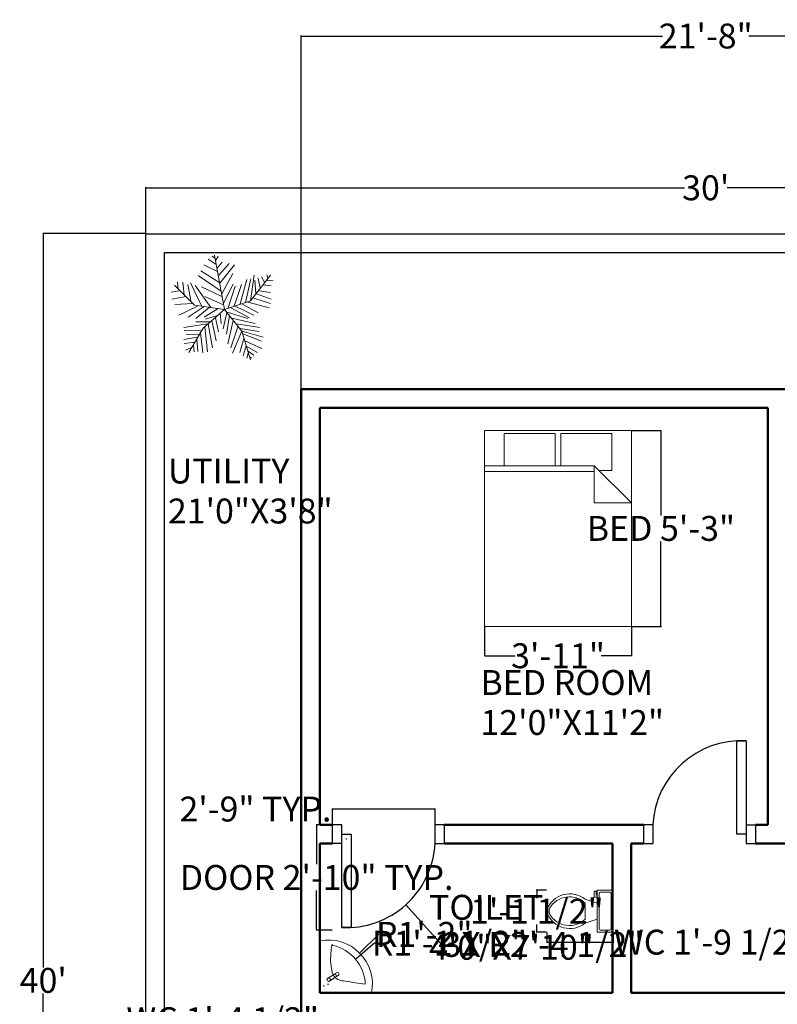
# Model space of a CAD drawing. Units: inches. Extents: x -1912 to -1462, y -785 to -198.
# Tile 2 of 3: x -1912 to -1668, y -515 to -198. Entities that reach past the tile are written whole.
import ezdxf

# ---------------------------------------------------------------- set-up
doc = ezdxf.new("R2010")
doc.units = ezdxf.units.IN
doc.header["$MEASUREMENT"] = 0
for name, color, linetype, lineweight in [('A-ANNO-DIMS', 2, 'Continuous', 18), ('A-AREA-IDEN', 7, 'Continuous', 18), ('A-DOOR', 4, 'Continuous', 25), ('A-FLOR-FIXT', 8, 'Continuous', 18), ('A-FURN', 8, 'Continuous', 18), ('A-WALL', 7, 'Continuous', 50), ('C-PROP', 8, 'Continuous', 25), ('L-PLNT-TREE', 3, 'Continuous', 13)]:
    doc.layers.add(name, color=color, linetype=linetype, lineweight=lineweight)
doc.styles.get("Standard").update_dxf_attribs({"font": 'arial.ttf'})
doc.dimstyles.get("Standard").update_dxf_attribs({"dimtxt": 8, "dimasz": 0.18, "dimexe": 0.18, "dimexo": 0.0625, "dimgap": 0.09, "dimtad": 0, "dimtih": 1, "dimtoh": 1, "dimzin": 0, "dimdsep": 46, "dimlunit": 3, "dimtxsty": 'Standard', "dimcen": 0.09, "dimadec": 0, "dimazin": 0, "dimtfac": 1, "dimtofl": 0, "dimtmove": 0, "dimatfit": 3, "dimfxl": 1, "dimtolj": 1, "dimtzin": 0, "dimarcsym": 0})

# ---------------------------------------------------------------- blocks, each defined once
blk = doc.blocks.new('Bed - Queen')
for p, q in [((0, -80.00003), (0, 0)), ((0, 0), (59.99999, 0)), ((59.99999, 0), (59.99999, -80.00003)), ((7.99999, -1.2), (28.79998, -1.2)), ((7.99999, -14.4), (7.99999, -1.2)), ((28.79998, -1.2), (28.79998, -14.4)), ((31.19999, -1.2), (51.99999, -1.2)), ((31.19999, -14.4), (31.19999, -1.2)), ((51.99999, -1.2), (51.99999, -16.4)), ((0, -14.4), (44.8, -14.4)), ((59.99999, -29.6), (44.8, -14.4)), ((44.8, -14.4), (44.8, -29.6)), ((44.8, -16.8), (0, -16.8)), ((51.99999, -16.4), (46.79936, -16.4)), ((44.8, -29.6), (59.99999, -29.6)), ((59.99999, -80.00003), (0, -80.00003))]:
    blk.add_line(p, q)
blk = doc.blocks.new('Toilet - top')
for p, q in [((9.5, -6), (9.5, -2)), ((-10, -8.5), (-8, -8.5)), ((-10, -9.5), (-10, -8.5)), ((-7, -9.5), (-10, -9.5)), ((-8, -8.5), (-8, -8)), ((-7, -8), (-7, -9.5)), ((-4, -8), (-6, -14)), ((4, -8), (6, -14)), ((4, -14), (-4, -14))]:
    blk.add_line(p, q)
blk.add_lwpolyline([(10.5, -8), (10.5, 0), (-10.5, 0), (-10.5, -8)], close=True)
for points in [[(-9.5, -2), (-9.5, -6)], [(8.5, -1), (-8.5, -1)], [(-8.5, -7), (8.5, -7)]]:
    blk.add_lwpolyline(points)
for centre, radius, start, end in [((-8.62, -1.88), 0.884, 81.8699, 188.1301), ((8.62, -1.88), 0.884, 351.8699, 98.1301), ((-8.62, -6.12), 0.884, 171.8699, 278.1301), ((8.62, -6.12), 0.884, 261.8699, 8.1301), ((3.52, -21.58), 12.17, 141.4691, 247.9714), ((4.2, -21.82), 11.33, 136.3677, 238.9468), ((-3.52, -21.58), 12.17, 292.0284, 38.5307), ((-4.2, -21.82), 11.33, 301.053, 43.6321), ((0, -27.88), 4, 245.7318, 294.2682), ((0, -29), 4, 254.8605, 285.1395)]:
    blk.add_arc(centre, radius, start, end)
blk = doc.blocks.new('*U11')
for p, q in [((-8.737, 47.138), (-17.069, 52.711)), ((-10.186, 53.64), (-13.084, 55.962)), ((0, 0), (-10.5, 57)), ((-9.099, 51.782), (-6.563, 55.962)), ((-7.288, 39.707), (-21.778, 46.673)), ((-7.65, 43.423), (-2.578, 49.46)), ((-5.839, 35.992), (4.667, 48.067)), ((-5.114, 27.632), (10.463, 46.673)), ((-3.665, 19.273), (-27.574, 35.527)), ((-5.114, 28.097), (-24.676, 40.636)), ((-2.941, 16.486), (8.652, 37.85)), ((16.259, 5.805), (23.142, 31.348)), ((22.055, 7.198), (27.489, 32.277)), ((27, 9), (48, 36)), ((27.127, 9.056), (31.112, 35.992)), ((35.096, 32.741), (37.27, 22.524)), ((38.719, 34.134), (41.979, 28.561)), ((44.153, 36.456), (45.239, 32.741)), ((-31.5, 4.5), (-52.5, 25.5)), ((-48.585, 21.131), (-49.309, 29.026)), ((-43.513, 28.561), (-42.427, 15.558)), ((-38.442, 26.239), (-34.819, 7.663)), ((-35.544, 28.097), (-24.314, 3.947)), ((-14.533, 2.09), (-30.834, 25.31)), ((-24.314, 23.917), (-2.941, 13.7)), ((-1.129, 6.734), (9.014, 26.704)), ((3.942, 1.625), (11.187, 24.381)), ((10.101, 3.483), (17.708, 26.239)), ((31.836, 30.883), (32.561, 16.486)), ((40.53, 25.775), (48.862, 24.846)), ((43.791, 29.954), (51.036, 30.883)), ((-47.498, 19.737), (-55.83, 18.344)), ((-40.615, 13.7), (-55.105, 10.913)), ((-20.691, 13.7), (-1.129, 4.876)), ((29.662, 12.307), (48.137, 6.269)), ((33.285, 16.486), (48.862, 10.913)), ((36.183, 19.737), (48.137, 17.88)), ((-33.37, 6.269), (-52.207, 5.34)), ((-28.299, 3.483), (-47.86, -5.805)), ((-21.416, 3.018), (-38.079, -8.128)), ((0, 0), (-31.5, 4.5)), ((-15.982, 2.09), (-30.11, -9.521)), ((0, 0), (-22.5, -19.5)), ((-6.563, 1.161), (-21.416, -8.128)), ((0, 0), (27, 9)), ((0, 0), (18, -22.5)), ((6.478, 1.625), (26.04, -8.592)), ((11.187, 3.483), (30.749, -5.805)), ((18.07, 5.805), (35.096, -3.483)), ((24.229, 7.663), (46.688, 1.625)), ((-6.563, -5.805), (-19.967, -9.985)), ((-9.461, -8.592), (-6.201, -23.453)), ((-4.752, -3.483), (-3.665, -14.629)), ((2.493, -3.019), (-1.491, -20.202)), ((1.769, -2.555), (24.229, -9.521)), ((5.029, -6.27), (2.131, -25.775)), ((7.565, -9.056), (32.198, -14.629)), ((-17.431, -15.094), (-42.789, -18.809)), ((-22.5, -19.5), (-37.5, -45)), ((-15.257, -12.772), (-30.11, -12.772)), ((-20.691, -18.345), (-17.793, -44.352)), ((-17.069, -15.094), (-12.721, -40.172)), ((-13.446, -11.378), (-8.737, -32.741)), ((9.014, -11.378), (3.58, -35.992)), ((14.085, -16.951), (6.478, -40.172)), ((12.274, -15.094), (36.907, -18.809)), ((16.259, -19.738), (36.183, -22.989)), ((-28.299, -29.026), (-42.789, -31.348)), ((-24.314, -21.596), (-42.427, -22.06)), ((-26.849, -26.24), (-40.253, -25.775)), ((-29.023, -30.884), (-27.936, -43.887)), ((-25.038, -23.918), (-22.865, -45.281)), ((18.07, -22.524), (8.289, -45.745)), ((20.244, -30.419), (15.897, -44.816)), ((18, -22.5), (27, -52.5)), ((18.433, -22.524), (40.53, -29.026)), ((19.157, -25.311), (38.719, -33.206)), ((-30.834, -34.135), (-42.427, -35.528)), ((-34.457, -39.708), (-40.978, -42.494)), ((-32.646, -36.921), (-31.921, -44.352)), ((22.78, -37.85), (19.519, -48.532)), ((21.331, -32.741), (39.081, -40.636)), ((22.78, -38.314), (34.372, -44.816)), ((24.591, -45.745), (23.142, -50.854)), ((24.591, -43.423), (30.749, -47.603)), ((26.764, -49.925), (28.213, -50.854))]:
    blk.add_line(p, q)
blk = doc.blocks.new('*D12')
at = {"layer": 'A-ANNO-DIMS', "color": 0, "lineweight": -2, "transparency": 16777216}
for p, q in [((-1871.08, -267.18), (-1871.08, -252.32)), ((-1870.9, -252.5), (-1697.95, -252.5)), ((-1511.26, -252.5), (-1684.2, -252.5)), ((-1511.08, -267.18), (-1511.08, -252.32))]:
    blk.add_line(p, q, dxfattribs=at)
at = {"layer": 'A-ANNO-DIMS', "color": 0, "transparency": 16777216}
for points in [[(-1870.9, -252.47), (-1870.9, -252.53), (-1871.08, -252.5)], [(-1511.26, -252.47), (-1511.26, -252.53), (-1511.08, -252.5)]]:
    blk.add_solid(points, dxfattribs=at)
at = {"layer": 'Defpoints', "color": 0, "transparency": 16777216}
for p in [(-1511.08, -252.5), (-1871.08, -267.24), (-1511.08, -267.24)]:
    blk.add_point(p, dxfattribs=at)
at = {"layer": 'A-ANNO-DIMS', "color": 0, "transparency": 16777216, "insert": (-1691.08, -252.5), "char_height": 8, "attachment_point": 5}
blk.add_mtext("\\A1;30'", dxfattribs=at)
blk = doc.blocks.new('*D13')
at = {"layer": 'A-ANNO-DIMS', "color": 0, "lineweight": -2, "transparency": 16777216}
for p, q in [((-1871.14, -267.24), (-1904.18, -267.24)), ((-1904, -267.42), (-1904, -503.07)), ((-1904, -747.06), (-1904, -511.42)), ((-1871.14, -747.24), (-1904.18, -747.24))]:
    blk.add_line(p, q, dxfattribs=at)
at = {"layer": 'A-ANNO-DIMS', "color": 0, "transparency": 16777216}
for points in [[(-1904.03, -267.42), (-1903.97, -267.42), (-1904, -267.24)], [(-1904.03, -747.06), (-1903.97, -747.06), (-1904, -747.24)]]:
    blk.add_solid(points, dxfattribs=at)
at = {"layer": 'Defpoints', "color": 0, "transparency": 16777216}
for p in [(-1871.08, -267.24), (-1904, -747.24), (-1871.08, -747.24)]:
    blk.add_point(p, dxfattribs=at)
at = {"layer": 'A-ANNO-DIMS', "color": 0, "transparency": 16777216, "insert": (-1904, -507.24), "char_height": 8, "attachment_point": 5}
blk.add_mtext("\\A1;40'", dxfattribs=at)
blk = doc.blocks.new('DOOR-30IN-LEAF-HINGE-JAMB')
for p, q in [((0, 3), (0, -3)), ((0, 3), (3, 3)), ((3, 3), (3, -3)), ((0, -3), (3, -3))]:
    blk.add_line(p, q)
blk.add_lwpolyline([(0, 0), (-3, 0), (-3, 30), (0, 30)], close=True)
blk.add_arc((-1.5, 1.5), 28.54, 86.9872, 176.9872)
blk = doc.blocks.new('*D15')
at = {"layer": 'A-ANNO-DIMS', "color": 0, "lineweight": -2, "transparency": 16777216}
for p, q in [((-1811.14, -457.24), (-1816.33, -457.24)), ((-1816.15, -457.42), (-1816.15, -469.93)), ((-1816.15, -490.89), (-1816.15, -478.38)), ((-1811.14, -491.07), (-1816.33, -491.07))]:
    blk.add_line(p, q, dxfattribs=at)
at = {"layer": 'A-ANNO-DIMS', "color": 0, "transparency": 16777216}
for points in [[(-1816.18, -457.42), (-1816.12, -457.42), (-1816.15, -457.24)], [(-1816.18, -490.89), (-1816.12, -490.89), (-1816.15, -491.07)]]:
    blk.add_solid(points, dxfattribs=at)
at = {"layer": 'Defpoints', "color": 0, "transparency": 16777216}
for p in [(-1811.08, -457.24), (-1816.15, -491.07), (-1811.08, -491.07)]:
    blk.add_point(p, dxfattribs=at)
at = {"layer": 'A-ANNO-DIMS', "color": 0, "transparency": 16777216, "insert": (-1816.15, -474.16), "char_height": 8, "attachment_point": 5}
blk.add_mtext('\\A1;DOOR 2\'-10" TYP.', dxfattribs=at)
blk = doc.blocks.new('*D16')
at = {"layer": 'A-ANNO-DIMS', "color": 0, "lineweight": -2, "transparency": 16777216}
for p, q in [((-1811.08, -452.17), (-1811.26, -452.17)), ((-1811.08, -457.18), (-1811.08, -451.99)), ((-1778.26, -452.17), (-1810.9, -452.17)), ((-1778.08, -457.18), (-1778.08, -451.99))]:
    blk.add_line(p, q, dxfattribs=at)
at = {"layer": 'A-ANNO-DIMS', "color": 0, "transparency": 16777216}
for points in [[(-1810.9, -452.14), (-1810.9, -452.2), (-1811.08, -452.17)], [(-1778.26, -452.14), (-1778.26, -452.2), (-1778.08, -452.17)]]:
    blk.add_solid(points, dxfattribs=at)
at = {"layer": 'Defpoints', "color": 0, "transparency": 16777216}
for p in [(-1811.08, -452.17), (-1811.08, -457.24), (-1778.08, -457.24)]:
    blk.add_point(p, dxfattribs=at)
at = {"layer": 'A-ANNO-DIMS', "color": 0, "transparency": 16777216, "insert": (-1835.8, -452.17), "char_height": 8, "attachment_point": 5}
blk.add_mtext('\\A1;2\'-9" TYP.', dxfattribs=at)
blk = doc.blocks.new('*D17')
at = {"layer": 'A-ANNO-DIMS', "color": 0, "lineweight": -2, "transparency": 16777216}
for p, q in [((-1742.16, -491.83), (-1742.16, -495.14)), ((-1720.86, -491.83), (-1720.86, -495.14)), ((-1741.98, -494.96), (-1721.04, -494.96)), ((-1720.86, -494.96), (-1720.68, -494.96))]:
    blk.add_line(p, q, dxfattribs=at)
at = {"layer": 'A-ANNO-DIMS', "color": 0, "transparency": 16777216}
for points in [[(-1741.98, -494.93), (-1741.98, -494.99), (-1742.16, -494.96)], [(-1721.04, -494.93), (-1721.04, -494.99), (-1720.86, -494.96)]]:
    blk.add_solid(points, dxfattribs=at)
at = {"layer": 'Defpoints', "color": 0, "transparency": 16777216}
for p in [(-1742.16, -491.77), (-1720.86, -491.77), (-1720.86, -494.96)]:
    blk.add_point(p, dxfattribs=at)
at = {"layer": 'A-ANNO-DIMS', "color": 0, "transparency": 16777216, "insert": (-1689.61, -494.96), "char_height": 8, "attachment_point": 5}
blk.add_mtext('\\A1;WC 1\'-9 1/2"', dxfattribs=at)
blk = doc.blocks.new('*D18')
at = {"layer": 'A-ANNO-DIMS', "color": 0, "lineweight": -2, "transparency": 16777216}
for p, q in [((-1742.22, -478.23), (-1745.53, -478.23)), ((-1745.35, -478.41), (-1745.35, -480.77)), ((-1745.35, -491.59), (-1745.35, -489.23)), ((-1742.22, -491.77), (-1745.53, -491.77))]:
    blk.add_line(p, q, dxfattribs=at)
at = {"layer": 'A-ANNO-DIMS', "color": 0, "transparency": 16777216}
for points in [[(-1745.38, -478.41), (-1745.32, -478.41), (-1745.35, -478.23)], [(-1745.38, -491.59), (-1745.32, -491.59), (-1745.35, -491.77)]]:
    blk.add_solid(points, dxfattribs=at)
at = {"layer": 'Defpoints', "color": 0, "transparency": 16777216}
for p in [(-1742.16, -478.23), (-1745.35, -491.77), (-1742.16, -491.77)]:
    blk.add_point(p, dxfattribs=at)
at = {"layer": 'A-ANNO-DIMS', "color": 0, "transparency": 16777216, "insert": (-1745.35, -485), "char_height": 8, "attachment_point": 5}
blk.add_mtext('\\A1;1\'-1 1/2"', dxfattribs=at)
blk = doc.blocks.new('*D19')
at = {"layer": 'A-ANNO-DIMS', "color": 0, "lineweight": -2, "transparency": 16777216}
for p, q in [((-1815.08, -519.88), (-1815.26, -519.88)), ((-1815.08, -522.26), (-1815.08, -519.7)), ((-1798.96, -519.88), (-1814.9, -519.88)), ((-1798.78, -522.26), (-1798.78, -519.7))]:
    blk.add_line(p, q, dxfattribs=at)
at = {"layer": 'A-ANNO-DIMS', "color": 0, "transparency": 16777216}
for points in [[(-1814.9, -519.85), (-1814.9, -519.91), (-1815.08, -519.88)], [(-1798.96, -519.85), (-1798.96, -519.91), (-1798.78, -519.88)]]:
    blk.add_solid(points, dxfattribs=at)
at = {"layer": 'Defpoints', "color": 0, "transparency": 16777216}
for p in [(-1815.08, -519.88), (-1815.08, -522.32), (-1798.78, -522.32)]:
    blk.add_point(p, dxfattribs=at)
at = {"layer": 'A-ANNO-DIMS', "color": 0, "transparency": 16777216, "insert": (-1846.33, -519.88), "char_height": 8, "attachment_point": 5}
blk.add_mtext('\\A1;WC 1\'-4 1/2"', dxfattribs=at)
blk = doc.blocks.new('*D29')
at = {"layer": 'A-ANNO-DIMS', "color": 0, "lineweight": -2, "transparency": 16777216}
for p, q in [((-1714.88, -330.48), (-1705.31, -330.48)), ((-1705.49, -330.66), (-1705.49, -357.79)), ((-1705.49, -393.28), (-1705.49, -366.15)), ((-1714.88, -393.46), (-1705.31, -393.46))]:
    blk.add_line(p, q, dxfattribs=at)
at = {"layer": 'A-ANNO-DIMS', "color": 0, "transparency": 16777216}
for points in [[(-1705.52, -330.66), (-1705.46, -330.66), (-1705.49, -330.48)], [(-1705.52, -393.28), (-1705.46, -393.28), (-1705.49, -393.46)]]:
    blk.add_solid(points, dxfattribs=at)
at = {"layer": 'Defpoints', "color": 0, "transparency": 16777216}
for p in [(-1714.94, -330.48), (-1705.49, -330.48), (-1714.94, -393.46)]:
    blk.add_point(p, dxfattribs=at)
at = {"layer": 'A-ANNO-DIMS', "color": 0, "transparency": 16777216, "insert": (-1705.49, -361.97), "char_height": 8, "attachment_point": 5}
blk.add_mtext('\\A1;BED 5\'-3"', dxfattribs=at)
blk = doc.blocks.new('*D30')
at = {"layer": 'A-ANNO-DIMS', "color": 0, "lineweight": -2, "transparency": 16777216}
for p, q in [((-1762.17, -393.52), (-1762.17, -403.08)), ((-1714.94, -393.52), (-1714.94, -403.08)), ((-1761.99, -402.9), (-1752.38, -402.9)), ((-1715.12, -402.9), (-1724.73, -402.9))]:
    blk.add_line(p, q, dxfattribs=at)
at = {"layer": 'A-ANNO-DIMS', "color": 0, "transparency": 16777216}
for points in [[(-1761.99, -402.87), (-1761.99, -402.93), (-1762.17, -402.9)], [(-1715.12, -402.87), (-1715.12, -402.93), (-1714.94, -402.9)]]:
    blk.add_solid(points, dxfattribs=at)
at = {"layer": 'Defpoints', "color": 0, "transparency": 16777216}
for p in [(-1762.17, -393.46), (-1714.94, -393.46), (-1714.94, -402.9)]:
    blk.add_point(p, dxfattribs=at)
at = {"layer": 'A-ANNO-DIMS', "color": 0, "transparency": 16777216, "insert": (-1738.55, -402.9), "char_height": 8, "attachment_point": 5}
blk.add_mtext('\\A1;3\'-11"', dxfattribs=at)
blk = doc.blocks.new('*D33')
at = {"layer": 'A-ANNO-DIMS', "color": 0, "lineweight": -2, "transparency": 16777216}
for p, q in [((-1821.08, -317.18), (-1821.08, -203.54)), ((-1820.9, -203.72), (-1704.98, -203.72)), ((-1561.26, -203.72), (-1677.18, -203.72)), ((-1561.08, -317.18), (-1561.08, -203.54))]:
    blk.add_line(p, q, dxfattribs=at)
at = {"layer": 'A-ANNO-DIMS', "color": 0, "transparency": 16777216}
for points in [[(-1820.9, -203.69), (-1820.9, -203.75), (-1821.08, -203.72)], [(-1561.26, -203.69), (-1561.26, -203.75), (-1561.08, -203.72)]]:
    blk.add_solid(points, dxfattribs=at)
at = {"layer": 'Defpoints', "color": 0, "transparency": 16777216}
for p in [(-1561.08, -203.72), (-1821.08, -317.24), (-1561.08, -317.24)]:
    blk.add_point(p, dxfattribs=at)
at = {"layer": 'A-ANNO-DIMS', "color": 0, "transparency": 16777216, "insert": (-1691.08, -203.72), "char_height": 8, "attachment_point": 5}
blk.add_mtext('\\A1;21\'-8"', dxfattribs=at)
blk = doc.blocks.new('*D44')
at = {"layer": 'A-ANNO-DIMS', "color": 0, "lineweight": -2, "transparency": 16777216}
for p, q in [((-1806.67, -461.74), (-1806.49, -461.74)), ((-1806.58, -461.83), (-1806.58, -461.65)), ((-1776.03, -495.68), (-1787.37, -483.09)), ((-1775.85, -495.68), (-1776.03, -495.68))]:
    blk.add_line(p, q, dxfattribs=at)
at = {"layer": 'A-ANNO-DIMS', "color": 0, "transparency": 16777216}
blk.add_solid([(-1787.34, -483.07), (-1787.39, -483.11), (-1787.49, -482.95)], dxfattribs=at)
at = {"layer": 'Defpoints', "color": 0, "transparency": 16777216}
for p in [(-1806.58, -461.74), (-1787.49, -482.95)]:
    blk.add_point(p, dxfattribs=at)
at = {"layer": 'A-ANNO-DIMS', "color": 0, "transparency": 16777216, "insert": (-1743.39, -495.68), "char_height": 8, "attachment_point": 5}
blk.add_mtext('\\A1;3X R2\'-4 1/2"', dxfattribs=at)
blk = doc.blocks.new('*D45')
at = {"layer": 'A-ANNO-DIMS', "color": 0, "lineweight": -2, "transparency": 16777216}
for p, q in [((-1796.28, -492.46), (-1802.2, -498.33)), ((-1796.1, -492.46), (-1796.28, -492.46)), ((-1812.5, -508.44), (-1812.32, -508.44)), ((-1812.41, -508.53), (-1812.41, -508.35))]:
    blk.add_line(p, q, dxfattribs=at)
at = {"layer": 'A-ANNO-DIMS', "color": 0, "transparency": 16777216}
blk.add_solid([(-1802.22, -498.3), (-1802.18, -498.35), (-1802.33, -498.45)], dxfattribs=at)
at = {"layer": 'Defpoints', "color": 0, "transparency": 16777216}
for p in [(-1802.33, -498.45), (-1812.41, -508.44)]:
    blk.add_point(p, dxfattribs=at)
at = {"layer": 'A-ANNO-DIMS', "color": 0, "transparency": 16777216, "insert": (-1781.55, -492.46), "char_height": 8, "attachment_point": 5}
blk.add_mtext('\\A1;R1\'-2"', dxfattribs=at)
blk = doc.blocks.new('*D46')
at = {"layer": 'A-ANNO-DIMS', "color": 0, "lineweight": -2, "transparency": 16777216}
for p, q in [((-1797.49, -495.31), (-1803.48, -500.34)), ((-1797.31, -495.31), (-1797.49, -495.31)), ((-1813.92, -509.03), (-1813.74, -509.03)), ((-1813.83, -509.12), (-1813.83, -508.94))]:
    blk.add_line(p, q, dxfattribs=at)
at = {"layer": 'A-ANNO-DIMS', "color": 0, "transparency": 16777216}
blk.add_solid([(-1803.5, -500.32), (-1803.46, -500.36), (-1803.61, -500.46)], dxfattribs=at)
at = {"layer": 'Defpoints', "color": 0, "transparency": 16777216}
for p in [(-1803.61, -500.46), (-1813.83, -509.03)]:
    blk.add_point(p, dxfattribs=at)
at = {"layer": 'A-ANNO-DIMS', "color": 0, "transparency": 16777216, "insert": (-1773.43, -495.31), "char_height": 8, "attachment_point": 5}
blk.add_mtext('\\A1;R1\'-1 1/2"', dxfattribs=at)

msp = doc.modelspace()

# ---------------------------------------------------------------- linework, layer by layer
at = {"layer": 'A-DOOR'}
for p, q in [((-1778.078, -463.241), (-1778.078, -457.241)), ((-1775.078, -457.241), (-1778.078, -457.241)), ((-1775.078, -463.241), (-1775.078, -457.241)), ((-1711.078, -457.241), (-1711.078, -463.241)), ((-1708.078, -457.241), (-1711.078, -457.241)), ((-1708.078, -457.241), (-1708.078, -463.241)), ((-1778.078, -463.241), (-1775.078, -463.241)), ((-1711.078, -463.241), (-1708.078, -463.241))]:
    msp.add_line(p, q, dxfattribs=at)
at = {"layer": 'A-FLOR-FIXT'}
for p, q in [((-1812.5, -506.5), (-1810, -505)), ((-1809, -505.5), (-1812, -507.5))]:
    msp.add_line(p, q, dxfattribs=at)
for centre in [(-1809.5, -505.25), (-1812.25, -507)]:
    msp.add_circle(centre, 0.559, dxfattribs=at)
for centre, radius, start, end in [((-1812.409, -508.436), 14.189, 348.59824, 100.84285), ((-1813.826, -509.034), 13.337, 2.2935, 77.76701)]:
    msp.add_arc(centre, radius, start, end, dxfattribs=at)
msp.add_open_spline([(-1800.5, -508.5), (-1802.616, -508.161), (-1805.958, -507.626), (-1813.262, -506.656), (-1811.098, -493.467), (-1811, -496)], degree=3, knots=[0, 0, 0, 0, 6.5764732, 10.3843598, 20.396852, 20.396852, 20.396852, 20.396852], dxfattribs=at)
at = {"layer": 'A-WALL'}
for p, q in [((-1821.078, -317.241), (-1561.078, -317.241)), ((-1821.078, -567.241), (-1821.078, -317.241)), ((-1815.078, -323.241), (-1671.078, -323.241)), ((-1815.078, -457.241), (-1815.078, -323.241)), ((-1671.078, -457.241), (-1671.078, -323.241)), ((-1815.078, -457.241), (-1811.078, -457.241)), ((-1775.078, -457.241), (-1711.078, -457.241)), ((-1675.078, -457.241), (-1671.078, -457.241)), ((-1815.078, -463.241), (-1811.078, -463.241)), ((-1815.078, -511.241), (-1815.078, -463.241)), ((-1775.078, -463.241), (-1721.078, -463.241)), ((-1721.078, -511.241), (-1721.078, -463.241)), ((-1715.078, -511.241), (-1715.078, -463.241)), ((-1715.078, -463.241), (-1711.078, -463.241)), ((-1675.078, -463.241), (-1665.078, -463.241)), ((-1815.078, -511.241), (-1721.078, -511.241)), ((-1715.078, -511.241), (-1613.799, -511.241))]:
    msp.add_line(p, q, dxfattribs=at)
at = {"layer": 'C-PROP'}
for p, q in [((-1865.078, -741.241), (-1865.078, -273.241)), ((-1865.078, -273.241), (-1517.078, -273.241))]:
    msp.add_line(p, q, dxfattribs=at)
msp.add_lwpolyline([(-1511.078, -747.241), (-1871.078, -747.241), (-1871.078, -267.241), (-1511.078, -267.241)], close=True, dxfattribs=at)

# ---------------------------------------------------------------- block references
at = {"layer": 'A-DOOR'}
msp.add_blockref('DOOR-30IN-LEAF-HINGE-JAMB', (-1678.078, -460.241), dxfattribs=at)
at = {"layer": 'A-DOOR', "rotation": 180}
msp.add_blockref('DOOR-30IN-LEAF-HINGE-JAMB', (-1808.078, -460.241), dxfattribs=at)
at = {"layer": 'A-FLOR-FIXT', "xscale": 0.6445682386841753, "yscale": 0.6445682386841753, "zscale": 0.6445682386841753, "rotation": 269.9999999999996}
msp.add_blockref('Toilet - top', (-1720.858, -485), dxfattribs=at)
at = {"layer": 'A-FURN', "xscale": 0.7872100769332117, "yscale": 0.7872100769332117, "zscale": 0.7872100769332117}
msp.add_blockref('Bed - Queen', (-1762.171, -330.481), dxfattribs=at)
at = {"layer": 'L-PLNT-TREE', "xscale": 0.307023879819639, "yscale": 0.307023879819639, "zscale": 0.307023879819639}
msp.add_blockref('*U11', (-1845.729, -291.627), dxfattribs=at)

# ---------------------------------------------------------------- texts
at = {"layer": 'A-AREA-IDEN'}
for s, p in [('UTILITY', (-1863.938, -347.529)), ('21\'0"X3\'8"', (-1863.938, -360.38)), ('BED ROOM', (-1763.5, -415.5)), ('12\'0"X11\'2"', (-1763.5, -428.351)), ('TOILET', (-1779.992, -487.755)), ('4\'0"X7\'10"', (-1779.992, -500.606))]:
    msp.add_text(s, height=8, dxfattribs=at).set_placement(p)

# ---------------------------------------------------------------- dimensions: what is measured, and where the dimension line sits
at = {"layer": 'A-ANNO-DIMS'}
for base, p1, p2, override, picture, middle in [((-1561.078, -203.718), (-1821.078, -317.241), (-1561.078, -317.241), {"dimdec": 1, "dimlfac": 1, "dimrnd": 0, "dimzin": 1, "dimdsep": 46, "dimlunit": 4, "dimfrac": 2}, '*D33', (-1691.078, -203.718)), ((-1511.078, -252.5), (-1871.078, -267.241), (-1511.078, -267.241), {"dimclrd": 0, "dimclre": 0, "dimclrt": 0}, '*D12', (-1691.078, -252.5)), ((-1714.938, -402.904), (-1762.171, -393.458), (-1714.938, -393.458), {"dimdec": 1, "dimlfac": 1, "dimrnd": 0, "dimzin": 1, "dimdsep": 46, "dimlunit": 4, "dimfrac": 2}, '*D30', (-1738.555, -402.904))]:
    dim = msp.add_linear_dim(base=base, p1=p1, p2=p2, dimstyle='Standard', override=override, dxfattribs=at)
    dim.commit()
    dim.dimension.update_dxf_attribs({"geometry": picture, "text_midpoint": middle})
for base, p1, p2, angle, override, picture, middle in [((-1904, -747.241), (-1871.078, -267.241), (-1871.078, -747.241), 90, {"dimclrd": 0, "dimclre": 0, "dimclrt": 0}, '*D13', (-1904, -507.241)), ((-1745.354, -491.768), (-1742.159, -478.232), (-1742.159, -491.768), 270, {"dimdec": 1, "dimlfac": 1, "dimrnd": 0, "dimzin": 1, "dimdsep": 46, "dimlunit": 4, "dimfrac": 2}, '*D18', (-1745.354, -485))]:
    dim = msp.add_linear_dim(base=base, p1=p1, p2=p2, angle=angle, dimstyle='Standard', override=override, dxfattribs=at)
    dim.commit()
    dim.dimension.update_dxf_attribs({"geometry": picture, "text_midpoint": middle})
for base, p1, p2, angle, text, picture, middle in [((-1705.492, -330.481), (-1714.938, -393.458), (-1714.938, -330.481), 90, 'BED <>', '*D29', (-1705.492, -361.969)), ((-1811.078, -452.167), (-1778.078, -457.241), (-1811.078, -457.241), 180, '<> TYP.', '*D16', (-1835.799, -452.167)), ((-1816.153, -491.069), (-1811.078, -457.241), (-1811.078, -491.069), 270, 'DOOR <> TYP.', '*D15', (-1816.153, -474.155)), ((-1815.078, -519.875), (-1798.777, -522.32), (-1815.078, -522.32), 180, 'WC <>', '*D19', (-1846.328, -519.875))]:
    dim = msp.add_linear_dim(base=base, p1=p1, p2=p2, angle=angle, text=text, dimstyle='Standard', override={"dimdec": 1, "dimlfac": 1, "dimrnd": 0, "dimzin": 1, "dimdsep": 46, "dimlunit": 4, "dimfrac": 2}, dxfattribs=at)
    dim.commit()
    dim.dimension.update_dxf_attribs({"geometry": picture, "text_midpoint": middle})
dim = msp.add_radius_dim(center=(-1806.578, -461.741), mpoint=(-1787.487, -482.954), text='3X <>', dimstyle='Standard', override={"dimdec": 1, "dimlfac": 1, "dimrnd": 0, "dimzin": 1, "dimdsep": 46, "dimlunit": 4, "dimfrac": 2}, dxfattribs=at)
dim.commit()
dim.dimension.update_dxf_attribs({"geometry": '*D44', "text_midpoint": (-1743.388, -495.682), "dimtype": 164})
dim = msp.add_linear_dim(base=(-1720.858, -494.963), p1=(-1742.159, -491.768), p2=(-1720.858, -491.768), text='WC <>', dimstyle='Standard', override={"dimdec": 1, "dimlfac": 1, "dimrnd": 0, "dimzin": 1, "dimdsep": 46, "dimlunit": 4, "dimfrac": 2}, dxfattribs=at)
dim.commit()
dim.dimension.update_dxf_attribs({"geometry": '*D17', "text_midpoint": (-1689.609, -494.963)})
for center, mpoint, picture, middle in [((-1813.826, -509.034), (-1803.614, -500.456), '*D46', (-1773.435, -495.309)), ((-1812.409, -508.436), (-1802.327, -498.452), '*D45', (-1781.546, -492.461))]:
    dim = msp.add_radius_dim(center=center, mpoint=mpoint, dimstyle='Standard', override={"dimdec": 1, "dimlfac": 1, "dimrnd": 0, "dimzin": 1, "dimdsep": 46, "dimlunit": 4, "dimfrac": 2}, dxfattribs=at)
    dim.commit()
    dim.dimension.update_dxf_attribs({"geometry": picture, "text_midpoint": middle, "dimtype": 164})

doc.saveas('drawing.dxf')
